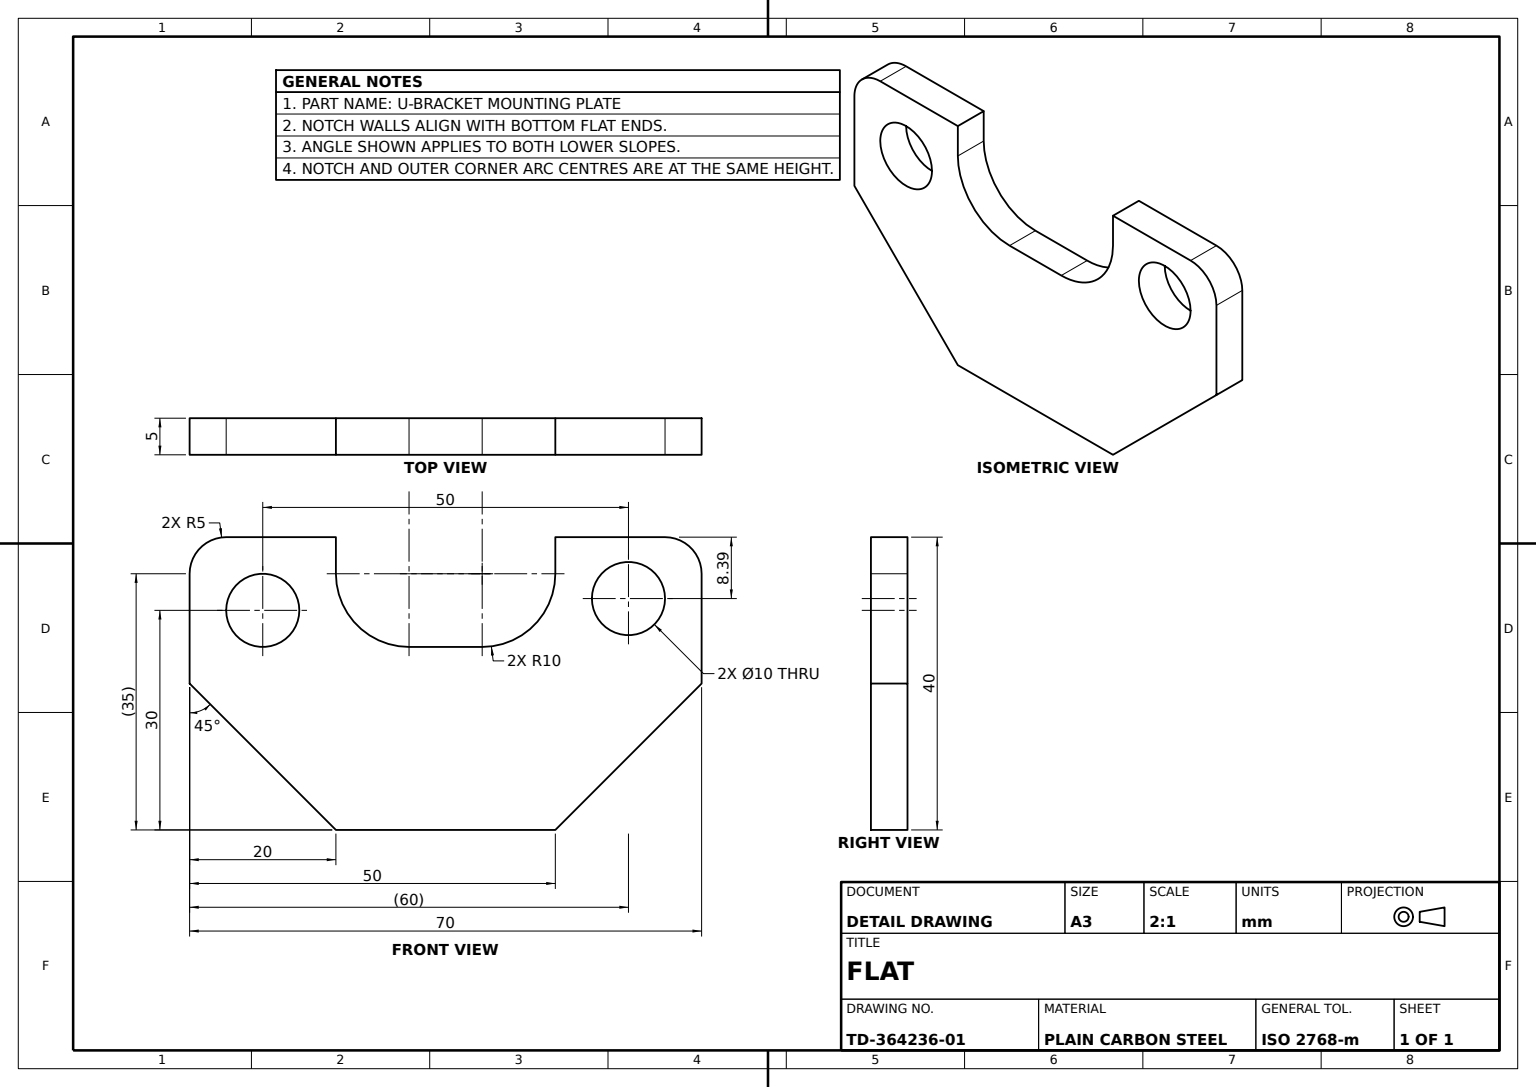
from build123d import *

# Parameters (mm, degrees)
BRACKET_PLATE_DEPTH      = 5
MOUNTING_HOLE_A_SKETCH_R = 5
MOUNTING_HOLE_A_10_DEPTH = 5
MOUNTING_HOLE_B_SKETCH_R = 5
MOUNTING_HOLE_B_10_DEPTH = 5
CORNER_FILLETS_R5_R      = 5


with BuildPart() as part:
    # Bracket Profile Sketch → Bracket Plate (new body)
    with BuildSketch(Plane.XY):
        with BuildLine():
            Line((0, 0), (30, 0))
            Line((30, 0), (50, 20))
            Line((50, 20), (50, 40))
            Line((50, 40), (30, 40))
            Line((30, 40), (30, 35))
            ThreePointArc((30, 35), (27.071067812, 27.928932188), (20, 25))
            Line((20, 25), (10, 25))
            ThreePointArc((10, 25), (2.928932188, 27.928932188), (0, 35))
            Line((0, 35), (0, 40))
            Line((0, 40), (-20, 40))
            Line((-20, 40), (-20, 20))
            Line((-20, 20), (0, 0))
        make_face()
    extrude(amount=BRACKET_PLATE_DEPTH)

    # Mounting Hole A Sketch → Mounting Hole A Ø10 (cut)
    with BuildSketch(Plane.XY.offset(5)):
        with Locations((-10, 30)):
            Circle(MOUNTING_HOLE_A_SKETCH_R)
    extrude(amount=-MOUNTING_HOLE_A_10_DEPTH, mode=Mode.SUBTRACT)

    # Mounting Hole B Sketch → Mounting Hole B Ø10 (cut)
    with BuildSketch(Plane.XY.offset(5)):
        with Locations((40, 31.609469521)):
            Circle(MOUNTING_HOLE_B_SKETCH_R)
    extrude(amount=-MOUNTING_HOLE_B_10_DEPTH, mode=Mode.SUBTRACT)

    # Corner Fillets R5
    corner_fillets_r5_edges = [part.edges().sort_by_distance(p)[0] for p in [
        (-20, 40, 2.5),
        (50, 40, 2.5),
    ]]
    fillet(corner_fillets_r5_edges, radius=CORNER_FILLETS_R5_R)


solid = part.part
